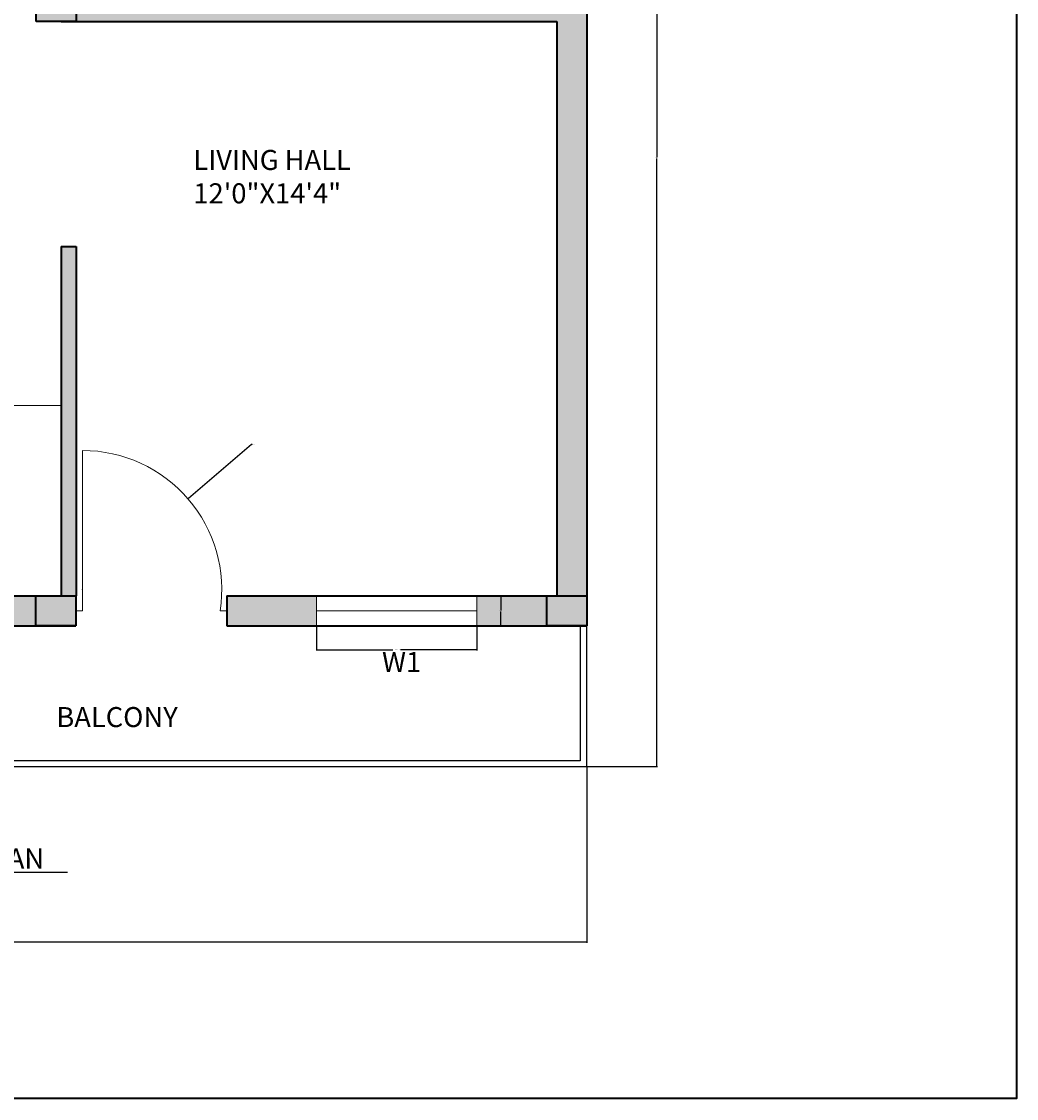
# Model space of a CAD drawing. Units: inches. Extents: x 1623 to 2200, y 2019 to 3010.
# Tile 3 of 6: x 1902 to 2200, y 2019 to 2342. Entities that reach past the tile are written whole.
import ezdxf

# ---------------------------------------------------------------- set-up
doc = ezdxf.new("R2010")
doc.units = ezdxf.units.IN
for name, color, linetype, lineweight in [('A-ANNO-DIMS', 2, 'Continuous', 18), ('A-ANNO-TITL', 7, 'Continuous', 25), ('A-ANNO-TTLB', 7, 'Continuous', 35), ('A-AREA-IDEN', 7, 'Continuous', 18), ('A-COLS', 7, 'Continuous', 40), ('A-DOOR', 3, 'Continuous', 18), ('A-FLOR-BALC', 7, 'Continuous', 25), ('A-FLOR-CASE', 8, 'Continuous', 18), ('A-GLAZ', 4, 'Continuous', 18), ('A-GLAZ-IDEN', 7, 'Continuous', 18), ('A-WALL', 7, 'Continuous', 35)]:
    doc.layers.add(name, color=color, linetype=linetype, lineweight=lineweight)
doc.layers.add('A-COLS-PATT', color=152, linetype='Continuous', lineweight=13, true_color=0x2776bb)
doc.layers.add('A-WALL-PATT', color=251, linetype='Continuous', lineweight=13, true_color=0x636466)
doc.styles.get("Standard").update_dxf_attribs({"font": 'arial.ttf'})
doc.dimstyles.get("Standard").update_dxf_attribs({"dimtxt": 0.18, "dimasz": 0.18, "dimexe": 0.18, "dimexo": 0.0625, "dimgap": 0.09, "dimtad": 0, "dimtih": 1, "dimtoh": 1, "dimdec": 4, "dimzin": 0, "dimdsep": 46, "dimtxsty": 'Standard', "dimcen": 0.09, "dimadec": 0, "dimazin": 0, "dimtfac": 1, "dimtdec": 4, "dimtofl": 0, "dimtmove": 0, "dimatfit": 3, "dimfxl": 1, "dimtolj": 1, "dimtzin": 0, "dimarcsym": 0})

# ---------------------------------------------------------------- blocks, each defined once
blk = doc.blocks.new('COL-12X9-PLAN')
for p, q in [((0, 0), (0, 9)), ((0, 9), (12, 9)), ((12, 9), (12, 0)), ((9, 0), (0, 0)), ((12, 0), (9, 0))]:
    blk.add_line(p, q)
blk = doc.blocks.new('WIN-48-PLAN')
for p, q in [((0, 9), (0, 0)), ((48, 4.5), (48, 9)), ((48, 9), (48, 0)), ((0, 0), (0, 4.5)), ((0, 4.5), (48, 4.5))]:
    blk.add_line(p, q)
blk = doc.blocks.new('*D14')
at = {"layer": 'A-ANNO-DIMS', "color": 0, "lineweight": -2, "transparency": 16777216}
for p, q in [((1990.33, 2160.96), (1990.33, 2153.64)), ((2038.33, 2160.96), (2038.33, 2153.64)), ((1990.51, 2153.82), (2013.21, 2153.82)), ((2038.15, 2153.82), (2015.44, 2153.82))]:
    blk.add_line(p, q, dxfattribs=at)
at = {"layer": 'A-ANNO-DIMS', "color": 0, "transparency": 16777216}
for points in [[(1990.51, 2153.85), (1990.51, 2153.79), (1990.33, 2153.82)], [(2038.15, 2153.85), (2038.15, 2153.79), (2038.33, 2153.82)]]:
    blk.add_solid(points, dxfattribs=at)
at = {"layer": 'Defpoints', "color": 0, "transparency": 16777216}
for p in [(1990.33, 2161.02), (2038.33, 2161.02), (2038.33, 2153.82)]:
    blk.add_point(p, dxfattribs=at)
at = {"layer": 'A-ANNO-DIMS', "color": 0, "transparency": 16777216, "insert": (2014.33, 2153.82), "char_height": 0.18, "attachment_point": 5}
blk.add_mtext('\\A1;WINDOW 48 TYP.', dxfattribs=at)
blk = doc.blocks.new('*D15')
at = {"layer": 'A-ANNO-DIMS', "color": 0, "lineweight": -2, "transparency": 16777216}
for p, q in [((2038.39, 2170.02), (2045.71, 2170.02)), ((2045.53, 2169.84), (2045.53, 2165.71)), ((2045.53, 2161.2), (2045.53, 2165.34)), ((2038.39, 2161.02), (2045.71, 2161.02))]:
    blk.add_line(p, q, dxfattribs=at)
at = {"layer": 'A-ANNO-DIMS', "color": 0, "transparency": 16777216}
for points in [[(2045.5, 2169.84), (2045.56, 2169.84), (2045.53, 2170.02)], [(2045.5, 2161.2), (2045.56, 2161.2), (2045.53, 2161.02)]]:
    blk.add_solid(points, dxfattribs=at)
at = {"layer": 'Defpoints', "color": 0, "transparency": 16777216}
for p in [(2038.33, 2170.02), (2045.53, 2170.02), (2038.33, 2161.02)]:
    blk.add_point(p, dxfattribs=at)
at = {"layer": 'A-ANNO-DIMS', "color": 0, "transparency": 16777216, "insert": (2045.53, 2165.52), "char_height": 0.18, "attachment_point": 5}
blk.add_mtext('\\A1;9 TYP.', dxfattribs=at)
blk = doc.blocks.new('*D28')
at = {"layer": 'A-ANNO-DIMS', "color": 0, "lineweight": -2, "transparency": 16777216}
for p, q in [((1710.33, 2118.83), (1710.33, 2066.05)), ((2071.33, 2118.83), (2071.33, 2066.05)), ((1710.51, 2066.23), (1890.55, 2066.23)), ((2071.15, 2066.23), (1891.1, 2066.23))]:
    blk.add_line(p, q, dxfattribs=at)
at = {"layer": 'A-ANNO-DIMS', "color": 0, "transparency": 16777216}
for points in [[(1710.51, 2066.26), (1710.51, 2066.2), (1710.33, 2066.23)], [(2071.15, 2066.26), (2071.15, 2066.2), (2071.33, 2066.23)]]:
    blk.add_solid(points, dxfattribs=at)
at = {"layer": 'Defpoints', "color": 0, "transparency": 16777216}
for p in [(1710.33, 2118.89), (2071.33, 2118.89), (2071.33, 2066.23)]:
    blk.add_point(p, dxfattribs=at)
at = {"layer": 'A-ANNO-DIMS', "color": 0, "transparency": 16777216, "insert": (1890.83, 2066.23), "char_height": 0.18, "attachment_point": 5}
blk.add_mtext('\\A1;361', dxfattribs=at)
blk = doc.blocks.new('*D29')
at = {"layer": 'A-ANNO-DIMS', "color": 0, "lineweight": -2, "transparency": 16777216}
for p, q in [((2071.39, 2483.53), (2092.46, 2483.53)), ((2092.28, 2483.35), (2092.28, 2301.39)), ((2092.28, 2119.07), (2092.28, 2301.03)), ((2071.39, 2118.89), (2092.46, 2118.89))]:
    blk.add_line(p, q, dxfattribs=at)
at = {"layer": 'A-ANNO-DIMS', "color": 0, "transparency": 16777216}
for points in [[(2092.25, 2483.35), (2092.31, 2483.35), (2092.28, 2483.53)], [(2092.25, 2119.07), (2092.31, 2119.07), (2092.28, 2118.89)]]:
    blk.add_solid(points, dxfattribs=at)
at = {"layer": 'Defpoints', "color": 0, "transparency": 16777216}
for p in [(2071.33, 2483.53), (2092.28, 2483.53), (2071.33, 2118.89)]:
    blk.add_point(p, dxfattribs=at)
at = {"layer": 'A-ANNO-DIMS', "color": 0, "transparency": 16777216, "insert": (2092.28, 2301.21), "char_height": 0.18, "attachment_point": 5}
blk.add_mtext('\\A1;364.64', dxfattribs=at)
blk = doc.blocks.new('*D60')
at = {"layer": 'A-ANNO-DIMS', "color": 0, "lineweight": -2, "transparency": 16777216}
for p, q in [((1970.84, 2215.29), (1952, 2199.11)), ((1971.02, 2215.29), (1970.84, 2215.29)), ((1920.14, 2171.83), (1920.32, 2171.83)), ((1920.23, 2171.74), (1920.23, 2171.92))]:
    blk.add_line(p, q, dxfattribs=at)
at = {"layer": 'A-ANNO-DIMS', "color": 0, "transparency": 16777216}
blk.add_solid([(1951.98, 2199.13), (1952.02, 2199.09), (1951.86, 2198.99)], dxfattribs=at)
at = {"layer": 'Defpoints', "color": 0, "transparency": 16777216}
for p in [(1951.86, 2198.99), (1920.23, 2171.83)]:
    blk.add_point(p, dxfattribs=at)
at = {"layer": 'A-ANNO-DIMS', "color": 0, "transparency": 16777216, "insert": (1971.5, 2215.29), "char_height": 0.18, "attachment_point": 5}
blk.add_mtext('\\A1;R41.69', dxfattribs=at)

msp = doc.modelspace()

# ---------------------------------------------------------------- hatches: boundary and pattern name
at = {"layer": 'A-COLS-PATT'}
h = msp.add_hatch(color=256, dxfattribs=at)
h.dxf.hatch_style = 1
h.paths.add_polyline_path([(1722.3258, 2483.5237), (1710.3258, 2483.5237), (1710.3258, 2474.5237), (1719.3258, 2474.5237), (1722.3258, 2474.5237)])
h.paths.add_polyline_path([(1809.3258, 2483.5237), (1797.3258, 2483.5237), (1797.3258, 2474.5237), (1806.3258, 2474.5237), (1809.3258, 2474.5237)])
h.paths.add_polyline_path([(1918.3972, 2483.5237), (1906.3972, 2483.5237), (1906.3972, 2474.5237), (1915.3972, 2474.5237), (1918.3972, 2474.5237)])
h.paths.add_polyline_path([(2071.3258, 2483.5237), (2059.3258, 2483.5237), (2059.3258, 2474.532), (2068.3258, 2474.532), (2071.3258, 2474.532)])
h.paths.add_polyline_path([(2071.3258, 2351.0312), (2059.3258, 2351.0312), (2059.3258, 2342.0312), (2068.3258, 2342.0312), (2071.3258, 2342.0312)])
h.paths.add_polyline_path([(1918.3258, 2351.0237), (1906.3258, 2351.0237), (1906.3258, 2342.0237), (1915.3258, 2342.0237), (1918.3258, 2342.0237)])
h.paths.add_polyline_path([(1722.3198, 2351.0237), (1710.3258, 2351.0237), (1710.3258, 2342.0237), (1719.3198, 2342.0237), (1722.3198, 2342.0237)])
h.paths.add_polyline_path([(1809.3158, 2351.0237), (1797.3258, 2351.0237), (1797.3258, 2346.5237), (1797.3158, 2342.0237), (1806.3158, 2342.0237), (1809.3158, 2342.0237)])
h.paths.add_polyline_path([(1722.3029, 2170.0237), (1710.3258, 2170.0237), (1710.3258, 2161.0237), (1714.3029, 2161.0237), (1719.3029, 2161.0237), (1722.3029, 2161.0237)])
h.paths.add_polyline_path([(1809.3258, 2170.0237), (1797.3258, 2170.0237), (1797.3258, 2161.0237), (1801.3258, 2161.0237), (1802.9141, 2161.0237), (1806.3258, 2161.0237), (1809.3258, 2161.0237)])
h.paths.add_polyline_path([(1918.2273, 2170.0237), (1906.2273, 2170.0237), (1906.2273, 2161.0237), (1915.2273, 2161.0237), (1918.2273, 2161.0237)])
h.paths.add_polyline_path([(2071.3258, 2170.0237), (2059.3258, 2170.0237), (2059.3258, 2161.0237), (2068.3258, 2161.0237), (2071.3258, 2161.0237)])
at = {"layer": 'A-WALL-PATT'}
h = msp.add_hatch(color=256, dxfattribs=at)
h.dxf.hatch_style = 1
h.paths.add_polyline_path([(1725.9857, 2483.5237), (1722.3258, 2483.5237), (1722.3258, 2474.5237), (1725.9857, 2474.5237), (1725.9857, 2479.0237)])
h.paths.add_polyline_path([(1797.3258, 2483.5237), (1749.9857, 2483.5237), (1749.9857, 2474.5237), (1797.3258, 2474.5237)])
h.paths.add_polyline_path([(1830.4977, 2483.5237), (1809.3258, 2483.5237), (1809.3258, 2474.5237), (1830.4977, 2474.5237), (1830.4977, 2479.0237)])
h.paths.add_polyline_path([(1906.3972, 2483.5237), (1878.4977, 2483.5237), (1878.4977, 2474.5237), (1906.3972, 2474.5237)])
h.paths.add_polyline_path([(1918.3258, 2474.5237), (1915.3972, 2474.5237), (1913.8258, 2474.5237), (1913.8258, 2395.0237), (1913.8258, 2384.7587), (1918.3258, 2384.7587), (1918.3258, 2395.0237)])
h.paths.add_polyline_path([(1801.8258, 2474.5237), (1797.3258, 2474.5237), (1797.3258, 2436.0951), (1801.8258, 2436.0951)], flags=17)
h.paths.add_polyline_path([(1719.3258, 2474.5237), (1710.3258, 2474.5237), (1710.3258, 2351.0237), (1719.3258, 2351.0237), (1719.3258, 2395.0237), (1801.8258, 2395.0237), (1801.8258, 2399.5237), (1719.3258, 2399.5237)])
h.paths.add_polyline_path([(1797.3158, 2346.5237), (1722.3198, 2346.5237), (1722.3198, 2342.0237), (1797.3158, 2342.0237)])
h.paths.add_polyline_path([(1801.8258, 2361.4421), (1797.3258, 2361.4421), (1797.3258, 2351.0237), (1801.8258, 2351.0237)], flags=17)
h.paths.add_polyline_path([(2059.3258, 2346.5237), (1918.3258, 2346.5237), (1918.3258, 2342.0237), (2059.3258, 2342.0237)])
h.paths.add_polyline_path([(1963.26, 2479.0237), (1963.26, 2483.5237), (1918.3972, 2483.5237), (1918.3972, 2474.5237), (1963.26, 2474.5237)])
h.paths.add_polyline_path([(2059.3258, 2483.5237), (2011.26, 2483.5237), (2011.26, 2474.5237), (2059.3258, 2474.5237)])
h.paths.add_polyline_path([(2071.3258, 2474.532), (2068.3258, 2474.532), (2062.3258, 2474.532), (2062.3258, 2351.0312), (2071.3258, 2351.0312)])
h.paths.add_polyline_path([(2071.3258, 2342.0312), (2068.3258, 2342.0312), (2062.3258, 2342.0312), (2062.3258, 2170.0237), (2071.3258, 2170.0237)])
h.paths.add_polyline_path([(2059.3258, 2170.0237), (2038.3258, 2170.0237), (2038.3258, 2161.0237), (2059.3258, 2161.0237)])
h.paths.add_polyline_path([(1990.3258, 2170.0237), (1963.4402, 2170.0237), (1963.4402, 2161.0237), (1990.3258, 2161.0237), (1990.3258, 2165.5237)])
h.paths.add_polyline_path([(1918.3258, 2274.595), (1913.8258, 2274.595), (1913.8258, 2170.0237), (1918.3258, 2170.0237)])
h.paths.add_polyline_path([(1906.2273, 2170.0237), (1871.454, 2170.0237), (1871.454, 2161.0237), (1906.2273, 2161.0237)])
h.paths.add_polyline_path([(1835.454, 2170.0237), (1809.3258, 2170.0237), (1809.3258, 2161.0237), (1835.454, 2161.0237), (1835.454, 2165.5237)])
h.paths.add_polyline_path([(1801.8258, 2270.095), (1865.2406, 2270.095), (1865.2406, 2274.595), (1797.3258, 2274.595), (1797.3258, 2170.0237), (1801.8258, 2170.0237)])
h.paths.add_polyline_path([(1719.3258, 2342.0237), (1719.3198, 2342.0237), (1710.3258, 2342.0237), (1710.3258, 2170.0237), (1719.3258, 2170.0237)])

# ---------------------------------------------------------------- linework, layer by layer
at = {"layer": 'A-ANNO-TITL'}
msp.add_line((1824.4388, 2087.1806), (1915.7543, 2087.1806), dxfattribs=at)
at = {"layer": 'A-ANNO-TTLB'}
msp.add_lwpolyline([(1623.0453, 3010.4913), (2200.0052, 3010.4913), (2200.0052, 2019.4245), (1623.0453, 2019.4245)], close=True, dxfattribs=at)
at = {"layer": 'A-DOOR'}
for p, q in [((1920.2273, 2165.5237), (1920.2273, 2213.5237)), ((1918.2273, 2165.5237), (1920.2273, 2165.5237)), ((1963.4402, 2165.5237), (1961.4402, 2165.5237))]:
    msp.add_line(p, q, dxfattribs=at)
msp.add_arc((1920.2273, 2171.8309), 41.6928, 351.298942, 90, dxfattribs=at)
at = {"layer": 'A-FLOR-BALC'}
for p, q in [((2071.3258, 2161.0237), (2069.3258, 2161.0237)), ((2069.3258, 2161.0237), (2069.3258, 2120.5833)), ((2071.3258, 2118.8921), (2071.3258, 2161.0237)), ((2071.3258, 2161.0237), (2071.3258, 2161.0237)), ((2069.3258, 2120.5833), (1801.3258, 2120.5833)), ((1714.8258, 2118.8921), (2071.3258, 2118.8921))]:
    msp.add_line(p, q, dxfattribs=at)
at = {"layer": 'A-FLOR-CASE'}
msp.add_line((1897.6607, 2227.0114), (1913.8258, 2227.0114), dxfattribs=at)
at = {"layer": 'A-WALL'}
for p, q in [((2071.3258, 2483.5237), (2071.3258, 2161.0237)), ((1913.8258, 2342.0237), (2062.3258, 2342.0237)), ((2062.3258, 2342.0237), (2062.3258, 2170.0237)), ((1913.8258, 2274.595), (1918.3258, 2274.595)), ((1913.8258, 2274.595), (1913.8258, 2170.0237)), ((1918.3258, 2274.595), (1918.3258, 2170.0237)), ((1801.8258, 2170.0237), (1913.8258, 2170.0237)), ((1963.4402, 2170.0237), (2062.3258, 2170.0237)), ((1963.4402, 2170.0237), (1963.4402, 2161.0237)), ((1797.3258, 2161.0237), (1918.2273, 2161.0237)), ((1963.4402, 2161.0237), (2071.3258, 2161.0237))]:
    msp.add_line(p, q, dxfattribs=at)

# ---------------------------------------------------------------- block references
at = {"layer": 'A-COLS'}
for p in [(1906.326, 2342.024), (1906.2275, 2161.024), (2059.326, 2161.024)]:
    msp.add_blockref('COL-12X9-PLAN', p, dxfattribs=at)
at = {"layer": 'A-GLAZ'}
msp.add_blockref('WIN-48-PLAN', (1990.326, 2161.024), dxfattribs=at)

# ---------------------------------------------------------------- texts
at = {"layer": 'A-ANNO-TITL', "insert": (1823.8511, 2094.305), "char_height": 6, "attachment_point": 1}
msp.add_mtext_dynamic_manual_height_columns('GROUND FLOOR PLAN', width=316.739638, gutter_width=12.5, heights=[0], dxfattribs=at)
at = {"layer": 'A-AREA-IDEN', "char_height": 6, "attachment_point": 1}
for s, width, insert in [('LIVING HALL\\P12\'0"X14\'4"', 125.509443, (1953.429, 2303.5652)), ('BALCONY', 174.905091, (1912.3689, 2136.6686))]:
    msp.add_mtext_dynamic_manual_height_columns(s, width=width, gutter_width=12.5, heights=[0], dxfattribs=dict(at, insert=insert))
at = {"layer": 'A-GLAZ-IDEN', "insert": (2009.9375, 2153.193), "char_height": 6, "attachment_point": 1}
msp.add_mtext_dynamic_manual_height_columns('W1', width=54.397259, gutter_width=12.5, heights=[0], dxfattribs=at)

# ---------------------------------------------------------------- dimensions: what is measured, and where the dimension line sits
at = {"layer": 'A-ANNO-DIMS'}
dim = msp.add_linear_dim(base=(2092.2758, 2483.532), p1=(2071.3258, 2118.8921), p2=(2071.3258, 2483.532), angle=90, dimstyle='Standard', override={"dimdec": 2, "dimlfac": 1, "dimrnd": 0, "dimzin": 0, "dimdsep": 46, "dimlunit": 2}, dxfattribs=at)
dim.commit()
dim.dimension.update_dxf_attribs({"geometry": '*D29', "text_midpoint": (2092.2758, 2301.212)})
dim = msp.add_radius_dim(center=(1920.2273, 2171.8309), mpoint=(1951.8599, 2198.9909), dimstyle='Standard', override={"dimdec": 2, "dimlfac": 1, "dimrnd": 0, "dimzin": 0, "dimdsep": 46, "dimlunit": 2}, dxfattribs=at)
dim.commit()
dim.dimension.update_dxf_attribs({"geometry": '*D60', "text_midpoint": (1971.4995, 2215.2869), "dimtype": 164})
dim = msp.add_linear_dim(base=(2045.5258, 2170.0237), p1=(2038.3258, 2161.0237), p2=(2038.3258, 2170.0237), angle=90, text='<> TYP.', dimstyle='Standard', override={"dimdec": 0, "dimlfac": 1, "dimrnd": 0, "dimzin": 0, "dimdsep": 46, "dimlunit": 2}, dxfattribs=at)
dim.commit()
dim.dimension.update_dxf_attribs({"geometry": '*D15', "text_midpoint": (2045.5258, 2165.5237)})
dim = msp.add_linear_dim(base=(2038.3258, 2153.8237), p1=(1990.3258, 2161.0237), p2=(2038.3258, 2161.0237), text='WINDOW <> TYP.', dimstyle='Standard', override={"dimdec": 0, "dimlfac": 1, "dimrnd": 0, "dimzin": 0, "dimdsep": 46, "dimlunit": 2}, dxfattribs=at)
dim.commit()
dim.dimension.update_dxf_attribs({"geometry": '*D14', "text_midpoint": (2014.3258, 2153.8237)})
dim = msp.add_linear_dim(base=(2071.3258, 2066.2306), p1=(1710.3258, 2118.8921), p2=(2071.3258, 2118.8921), dimstyle='Standard', override={"dimdec": 0, "dimlfac": 1, "dimrnd": 0, "dimzin": 0, "dimdsep": 46, "dimlunit": 2}, dxfattribs=at)
dim.commit()
dim.dimension.update_dxf_attribs({"geometry": '*D28', "text_midpoint": (1890.8258, 2066.2306)})

doc.saveas('drawing.dxf')
